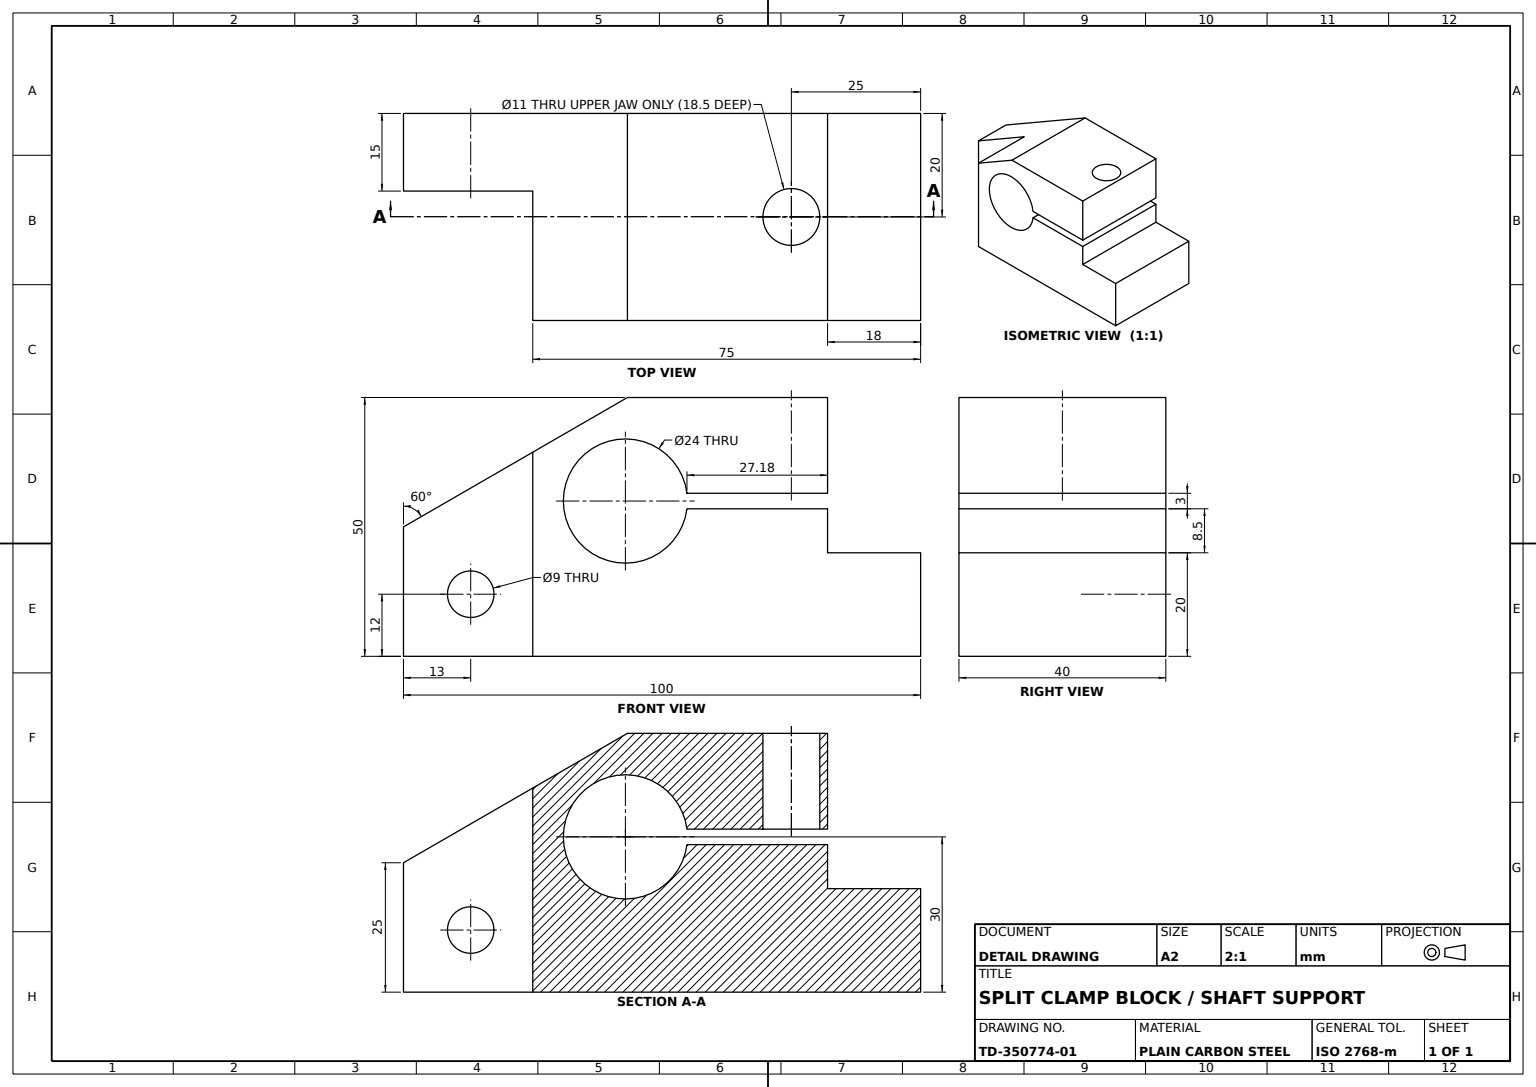
SolidWorks part; units mm, degrees
material "Plain Carbon Steel"
ref_plane "Front Plane" through (0, 0, 0) normal (0, 0, 1) x (1, 0, 0)
ref_plane "Top Plane" through (0, 0, 0) normal (0, 1, 0) x (1, 0, 0)
ref_plane "Right Plane" through (0, 0, 0) normal (1, 0, 0) x (0, 0, -1)
sketch "Block Profile Sketch" plane through (0, 0, 0) normal (0, 0, 1) x (1, 0, 0)
  line L0 (-58.3395, 25) -> (-58.3395, 0)
  line L1 (-58.3395, 0) -> (41.6605, 0)
  line L2 (41.6605, 0) -> (41.6605, 20)
  line L3 (41.6605, 20) -> (23.6605, 20)
  line L4 (23.6605, 20) -> (23.6605, 28.5)
  line L5 (23.6605, 28.5) -> (-3.5236, 28.5)
  line L6 (-58.3395, 25) -> (-15.0383, 50)
  line L7 (-3.5236, 31.5) -> (23.6605, 31.5)
  line L8 (23.6605, 31.5) -> (23.6605, 50)
  line L9 (-58.3395, 25) -> (-58.3395, 47.207) construction
  line L10 (-15.0383, 50) -> (23.6605, 50)
  arc A0 (-3.5236, 31.5) -> (-3.5236, 28.5) centre (-15.4295, 30) ccw
  circle A1 centre (-45.3395, 12) radius 4.5
  dimension "D7" = 24
  dimension "D10" = 9
  dimension "D1" = 100
  dimension "D2" = 20
  dimension "D3" = 50
  dimension "D4" = 25
  dimension "D5" = 18
  dimension "D6" = 60
  dimension "D8" = 13
  dimension "D9" = 12
  dimension "D11" = 58.3395
  dimension "D12" = 8.5
  dimension "D13" = 3
  dimension "D14" = 27.1841
extrude "Block Body" add sketch "Block Profile Sketch" along normal blind 40 contours L6 L10 L8 L7 A0 L5 L4 L3 L2 L1 L0
sketch "Cross Hole Sketch" plane through (0, 0, 40) normal (0, 0, 1) x (1, 0, 0)
  line L0 (-58.3395, 25) -> (-58.3395, 0) construction
  line L1 (-58.3395, 0) -> (41.6605, 0) construction
  circle A0 centre (-45.3395, 12) radius 4.5
  dimension "D3" = 9
  dimension "D1" = 13
  dimension "D2" = 12
extrude "Cross Hole" cut sketch "Cross Hole Sketch" against normal through all
sketch "Rectangular Cut Sketch" plane through (0, 0, 0) normal (0, -1, 0) x (1, 0, 0)
  line L0 (-58.3395, 40) -> (-58.3395, 0) construction
  line L1 (-58.3395, 15) -> (-33.3395, 15)
  line L2 (-58.3395, 15) -> (-58.3395, 40)
  line L3 (-58.3395, 40) -> (-33.3395, 40)
  line L4 (-33.3395, 15) -> (-33.3395, 40)
  line L5 (-58.3395, 40) -> (41.6605, 40) construction
  line L6 (-58.3395, 0) -> (41.6605, 0) construction
  line L7 (41.6605, 40) -> (41.6605, 0) construction
  dimension "D1" = 15
  dimension "D2" = 75
extrude "Rectangular Cut 15x75" cut sketch "Rectangular Cut Sketch" against normal through all
sketch "Top Clamp Hole Sketch" plane through (0, 50, 0) normal (0, 1, 0) x (1, 0, 0)
  line L0 (41.6605, -40) -> (41.6605, 0) construction
  line L2 (-15.0383, 0) -> (23.6605, 0) construction
  circle A0 centre (16.6605, -20) radius 5.5
  dimension "D2" = 11
  dimension "D1" = 25
  dimension "D3" = 20
extrude "Top Clamp Hole" cut sketch "Top Clamp Hole Sketch" against normal up to surface (18.5 mm away) up to face at (10.0684, 31.5, 20)
